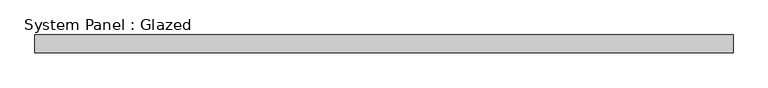
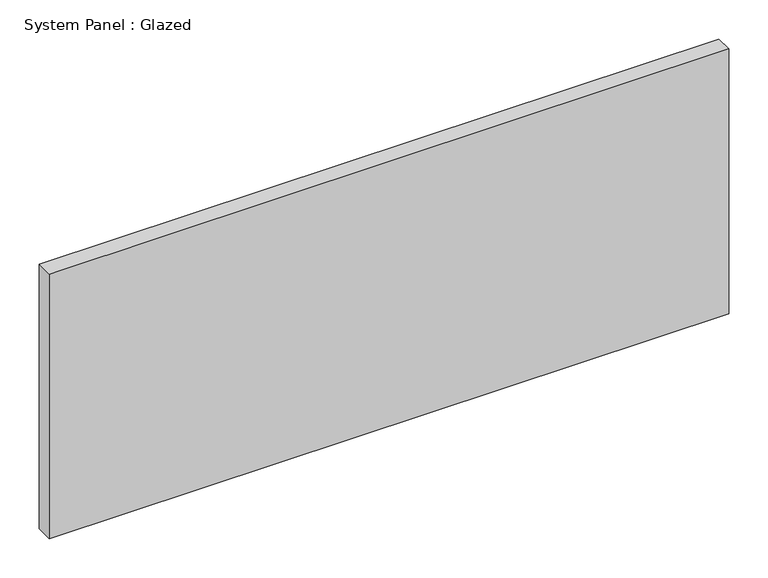
"""IFC4 building model written with IfcOpenShell, lengths in millimetres: plate geometry, System Panel : Glazed."""

from ifc_helpers import new_model, si_unit, origin, origin_with_axes, place, context, project, spatial, polyline, outline, extrude, source, transform, mapped, element, save


def system_panel_glazed_9d2fc6ec(model_context):
    return source(origin(), model_context, "Body", "SweptSolid", [
        extrude(outline(polyline([(501.65, 19.05), (-501.65, 19.05), (-501.65, 44.45), (501.65, 44.45), (501.65, 19.05)])), origin_with_axes(), (0.0, 0.0, 1.0), 412.75),
    ])


if __name__ == "__main__":
    model = new_model("IFC4")
    model_context = context("Model", 3, world=origin())
    ifc_project = project(units=[si_unit("LENGTHUNIT", "METRE", prefix="MILLI")], contexts=[model_context])
    site = spatial("IfcSite", under=ifc_project)
    building = spatial("IfcBuilding", under=site)
    placement = place(None, origin())
    system_panel_glazed_shape = system_panel_glazed_9d2fc6ec(model_context)
    element("IfcPlate", 1, ObjectType="System Panel : Glazed", at=placement, inside=building, context=model_context, shape_type="MappedRepresentation", body=[
        mapped(system_panel_glazed_shape, transform((0.0, 0.0, 0.0), x_axis=(1.0, 0.0, 0.0), y_axis=(0.0, 1.0, 0.0), z_axis=(0.0, 0.0, 1.0))),
    ])
    save(model, "model.ifc")

# Revit data of these elements
# Type "System Panel : Glazed"
#   Construction Type Id = "GSP4R"
#   Analytic Construction = "1/8 in Pilkington single glazing"
#   Visual Light Transmittance = 0.9
#   Solar Heat Gain Coefficient = 0.86
#   Heat Transfer Coefficient (U) = 1.18115 BTU/(h·ft²·°F)
#   Define Thermal Properties by = 1
# Element 1 (IfcPlate, "System Panel : Glazed")
#   Materials on its faces: "Glass"
# Materials
#   "Glass": class "Glass", colour RGB 0 128 192, transparency 0.75, Description = "Soda Lime Glass", Cost = 0
